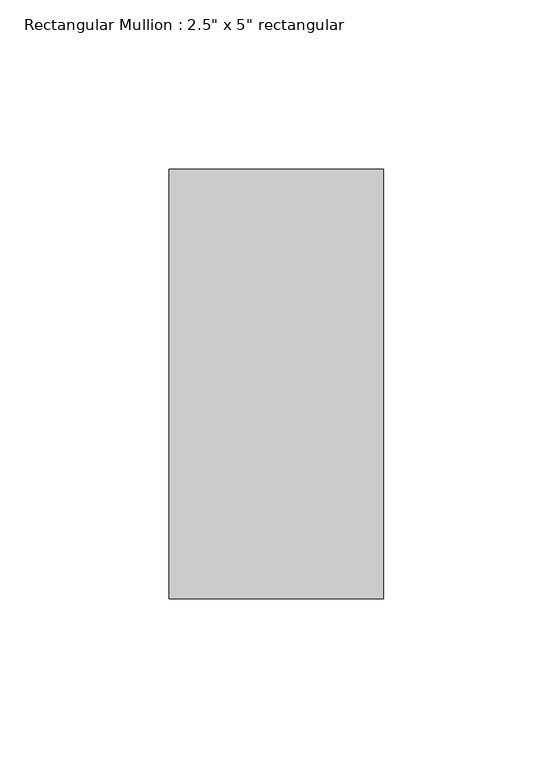
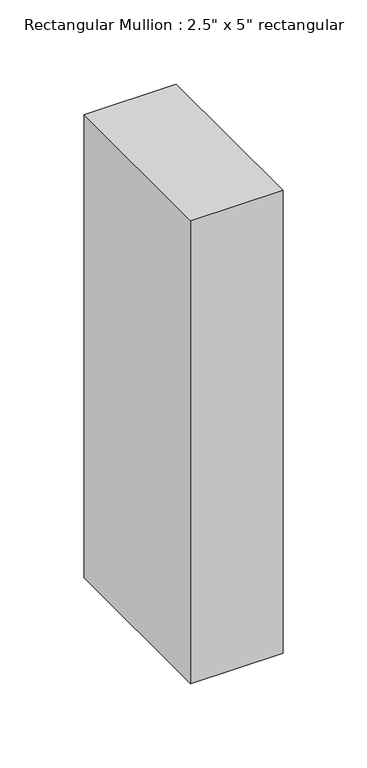
"""IFC4 building model written with IfcOpenShell, lengths in millimetres: member geometry."""

from ifc_helpers import new_model, si_unit, frame, origin, place, context, project, spatial, polyline, outline, extrude, source, transform, mapped, element, save


def member_80bb9b3a(model_context):
    return source(origin(), model_context, "Body", "SweptSolid", [
        extrude(outline(polyline([(31.75, 63.5), (31.75, -63.5), (-31.75, -63.5), (-31.75, 63.5), (31.75, 63.5)])), frame((0.0, 0.0, -336.55), z_axis=(0.0, 0.0, 1.0), x_axis=(1.0, 0.0, 0.0)), (0.0, 0.0, 1.0), 336.55),
    ])


if __name__ == "__main__":
    model = new_model("IFC4")
    model_context = context("Model", 3, world=origin())
    ifc_project = project(units=[si_unit("LENGTHUNIT", "METRE", prefix="MILLI")], contexts=[model_context])
    site = spatial("IfcSite", under=ifc_project)
    building = spatial("IfcBuilding", under=site)
    placement = place(None, origin())
    member_shape = member_80bb9b3a(model_context)
    element("IfcMember", 1, ObjectType="Rectangular Mullion : 2.5\" x 5\" rectangular", at=placement, inside=building, context=model_context, shape_type="MappedRepresentation", body=[
        mapped(member_shape, transform((0.0, 0.0, 0.0), x_axis=(1.0, 0.0, 0.0), y_axis=(0.0, 1.0, 0.0), z_axis=(0.0, 0.0, 1.0))),
    ])
    save(model, "model.ifc")

# Revit data of these elements
# Type "Rectangular Mullion : 2.5\" x 5\" rectangular"
#   built-in parameter 1007304 = 0.416667 (stored number, unit not read)
#   built-in parameter 1007301 = 0.104167 (stored number, unit not read)
#   built-in parameter 1007300 = 0.104167 (stored number, unit not read)
# Element 1 (IfcMember, "Rectangular Mullion : 2.5\" x 5\" rectangular")
#   Materials on its faces: "Aluminum"
# Materials
#   "Aluminum": class "Metal", colour RGB 247 247 247, transparency 0, Description = "Aluminum 6061", Cost = 0
